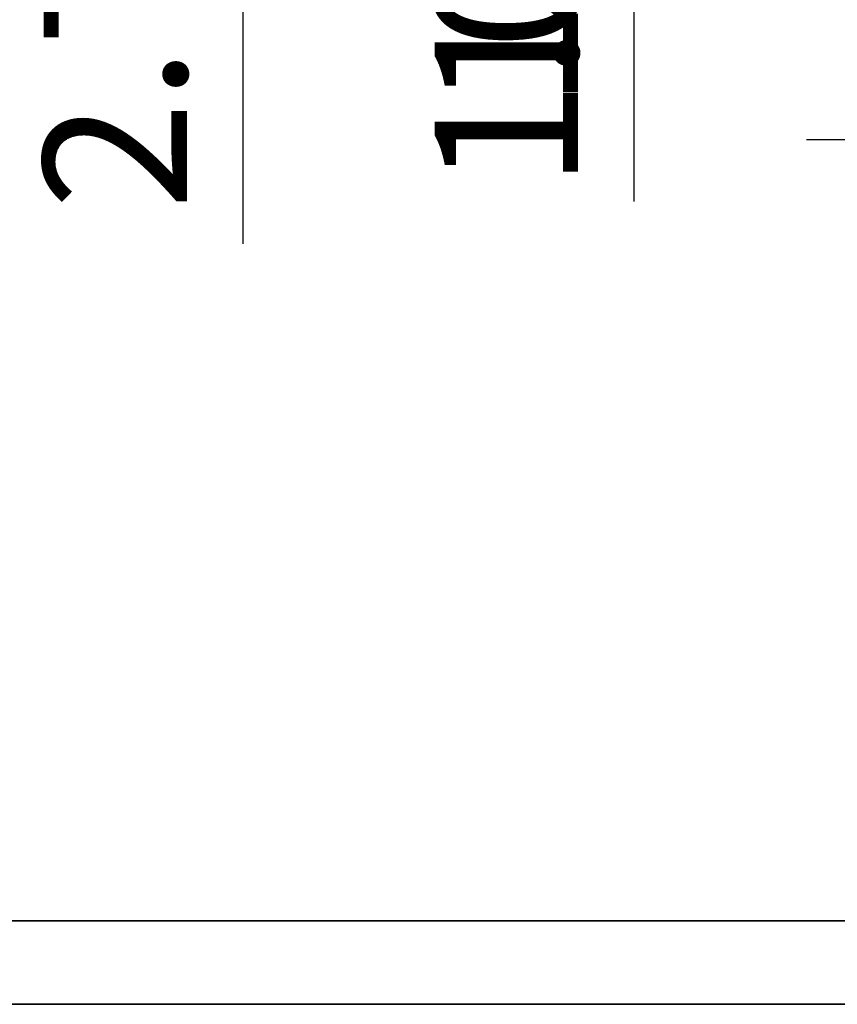
# Model space of a CAD drawing. Units: metres. Extents: x 782 to 1487, y 1262 to 7446.
# Tile 2 of 25: x 807.01 to 821.27, y 1262.35 to 1279.51. Entities that reach past the tile are written whole.
import ezdxf

# ---------------------------------------------------------------- set-up
doc = ezdxf.new("R2010")
doc.units = ezdxf.units.M
doc.layers.add('A-ANNO-DIMS', color=2, linetype='Continuous', lineweight=18)
doc.layers.add('A-ANNO-TTLB', color=7, linetype='Continuous', lineweight=35)
doc.styles.get("Standard").update_dxf_attribs({"font": 'arial.ttf'})
doc.dimstyles.new('ISO-25', dxfattribs={"dimtxt": 2.5, "dimasz": 2.5, "dimexe": 1.25, "dimexo": 0.625, "dimtad": 1, "dimtxsty": 'Standard', "dimcen": 2.5, "dimadec": 0, "dimazin": 0, "dimtfac": 1, "dimtmove": 0, "dimatfit": 3, "dimfxl": 1, "dimarcsym": 0})

# ---------------------------------------------------------------- blocks, each defined once
blk = doc.blocks.new('*D10')
at = {"layer": 'A-ANNO-DIMS', "color": 0, "lineweight": -2, "transparency": 16777216}
for p, q in [((825.73, 1277.527), (825.73, 1276.166)), ((826.753, 1277.552), (826.753, 1276.166)), ((823.23, 1277.416), (820.73, 1277.416)), ((825.73, 1277.416), (826.753, 1277.416)), ((829.253, 1277.416), (839.235, 1277.416))]:
    blk.add_line(p, q, dxfattribs=at)
at = {"layer": 'A-ANNO-DIMS', "color": 0, "transparency": 16777216}
for points in [[(823.23, 1277.833), (823.23, 1276.999), (825.73, 1277.416)], [(829.253, 1277.833), (829.253, 1276.999), (826.753, 1277.416)]]:
    blk.add_solid(points, dxfattribs=at)
at = {"layer": 'Defpoints', "color": 0, "transparency": 16777216}
for p in [(825.73, 1278.152), (826.753, 1278.177), (826.753, 1277.416)]:
    blk.add_point(p, dxfattribs=at)
at = {"layer": 'A-ANNO-DIMS', "color": 0, "transparency": 16777216, "insert": (835.494, 1279.543), "char_height": 2.5, "attachment_point": 5}
blk.add_mtext('1,02', dxfattribs=at)
blk = doc.blocks.new('*D62')
at = {"layer": 'A-ANNO-DIMS', "color": 0, "lineweight": -2, "transparency": 16777216}
for p, q in [((810.9, 1295.567), (810.9, 1298.067)), ((811.505, 1293.067), (809.65, 1293.067)), ((810.9, 1293.067), (810.9, 1290.305)), ((811.505, 1290.305), (809.65, 1290.305)), ((810.9, 1287.805), (810.9, 1275.602))]:
    blk.add_line(p, q, dxfattribs=at)
at = {"layer": 'A-ANNO-DIMS', "color": 0, "transparency": 16777216}
for points in [[(810.483, 1295.567), (811.317, 1295.567), (810.9, 1293.067)], [(810.483, 1287.805), (811.317, 1287.805), (810.9, 1290.305)]]:
    blk.add_solid(points, dxfattribs=at)
at = {"layer": 'Defpoints', "color": 0, "transparency": 16777216}
for p in [(812.13, 1293.067), (810.9, 1290.305), (812.13, 1290.305)]:
    blk.add_point(p, dxfattribs=at)
at = {"layer": 'A-ANNO-DIMS', "color": 0, "transparency": 16777216, "insert": (808.999, 1280.454), "char_height": 2.5, "attachment_point": 5, "rotation": 90}
blk.add_mtext('2.762', dxfattribs=at)
blk = doc.blocks.new('*D67')
at = {"layer": 'A-ANNO-DIMS', "color": 0, "lineweight": -2, "transparency": 16777216}
for p, q in [((817.721, 1296.199), (817.721, 1298.699)), ((817.205, 1293.699), (818.971, 1293.699)), ((817.721, 1293.699), (817.721, 1293.067)), ((817.205, 1293.067), (818.971, 1293.067)), ((817.721, 1290.567), (817.721, 1278.407))]:
    blk.add_line(p, q, dxfattribs=at)
at = {"layer": 'A-ANNO-DIMS', "color": 0, "transparency": 16777216}
for points in [[(817.304, 1296.199), (818.138, 1296.199), (817.721, 1293.699)], [(817.304, 1290.567), (818.138, 1290.567), (817.721, 1293.067)]]:
    blk.add_solid(points, dxfattribs=at)
at = {"layer": 'Defpoints', "color": 0, "transparency": 16777216}
for p in [(816.58, 1293.699), (816.58, 1293.067), (817.721, 1293.067)]:
    blk.add_point(p, dxfattribs=at)
at = {"layer": 'A-ANNO-DIMS', "color": 0, "transparency": 16777216, "insert": (815.819, 1283.237), "char_height": 2.5, "attachment_point": 5, "rotation": 90}
blk.add_mtext('0.632', dxfattribs=at)
blk = doc.blocks.new('*D68')
at = {"layer": 'A-ANNO-DIMS', "color": 0, "lineweight": -2, "transparency": 16777216}
for p, q in [((817.721, 1295.567), (817.721, 1298.067)), ((815.508, 1293.067), (818.971, 1293.067)), ((817.721, 1293.067), (817.721, 1291.686)), ((815.508, 1291.686), (818.971, 1291.686)), ((817.721, 1289.186), (817.721, 1277.718))]:
    blk.add_line(p, q, dxfattribs=at)
at = {"layer": 'A-ANNO-DIMS', "color": 0, "transparency": 16777216}
for points in [[(817.304, 1295.567), (818.138, 1295.567), (817.721, 1293.067)], [(817.304, 1289.186), (818.138, 1289.186), (817.721, 1291.686)]]:
    blk.add_solid(points, dxfattribs=at)
at = {"layer": 'Defpoints', "color": 0, "transparency": 16777216}
for p in [(814.883, 1293.067), (814.883, 1291.686), (817.721, 1291.686)]:
    blk.add_point(p, dxfattribs=at)
at = {"layer": 'A-ANNO-DIMS', "color": 0, "transparency": 16777216, "insert": (815.819, 1282.202), "char_height": 2.5, "attachment_point": 5, "rotation": 90}
blk.add_mtext('1.381', dxfattribs=at)
blk = doc.blocks.new('*D69')
at = {"layer": 'A-ANNO-DIMS', "color": 0, "lineweight": -2, "transparency": 16777216}
for p, q in [((817.721, 1294.186), (817.721, 1296.686)), ((815.508, 1291.686), (818.971, 1291.686)), ((817.721, 1291.686), (817.721, 1290.305)), ((815.508, 1290.305), (818.971, 1290.305)), ((817.721, 1287.805), (817.721, 1276.337))]:
    blk.add_line(p, q, dxfattribs=at)
at = {"layer": 'A-ANNO-DIMS', "color": 0, "transparency": 16777216}
for points in [[(817.304, 1294.186), (818.138, 1294.186), (817.721, 1291.686)], [(817.304, 1287.805), (818.138, 1287.805), (817.721, 1290.305)]]:
    blk.add_solid(points, dxfattribs=at)
at = {"layer": 'Defpoints', "color": 0, "transparency": 16777216}
for p in [(814.883, 1291.686), (814.883, 1290.305), (817.721, 1290.305)]:
    blk.add_point(p, dxfattribs=at)
at = {"layer": 'A-ANNO-DIMS', "color": 0, "transparency": 16777216, "insert": (815.819, 1280.821), "char_height": 2.5, "attachment_point": 5, "rotation": 90}
blk.add_mtext('1.381', dxfattribs=at)

msp = doc.modelspace()

# ---------------------------------------------------------------- linework, layer by layer
at = {"layer": 'A-ANNO-TTLB'}
for points in [[(787.4248, 1342.9861), (880.8003, 1342.9861), (880.8003, 1263.8004), (787.4248, 1263.8004)], [(883.6865, 1262.3458), (787.4248, 1262.3458), (787.4248, 1342.9861), (883.6865, 1342.9861)], [(788.8147, 1341.5907), (880.8003, 1341.5907), (880.8003, 1263.8004), (788.8147, 1263.8004)]]:
    msp.add_lwpolyline(points, close=True, dxfattribs=at)

# ---------------------------------------------------------------- dimensions: what is measured, and where the dimension line sits
at = {"layer": 'A-ANNO-DIMS'}
for base, p1, p2, picture, middle in [((817.7211, 1293.0674), (816.58, 1293.6994), (816.58, 1293.0674), '*D67', (815.8188, 1283.2371)), ((810.9, 1290.3053), (812.13, 1293.0674), (812.13, 1290.3053), '*D62', (808.9986, 1280.4536)), ((817.7211, 1291.6863), (814.8832, 1293.0674), (814.8832, 1291.6863), '*D68', (815.8188, 1282.2022)), ((817.7211, 1290.3053), (814.8832, 1291.6863), (814.8832, 1290.3053), '*D69', (815.8188, 1280.8211))]:
    dim = msp.add_linear_dim(base=base, p1=p1, p2=p2, angle=90, dimstyle='ISO-25', override={"dimdec": 3, "dimlfac": 1, "dimrnd": 0, "dimzin": 0, "dimdsep": 46, "dimlunit": 2}, dxfattribs=at)
    dim.commit()
    dim.dimension.update_dxf_attribs({"geometry": picture, "text_midpoint": middle})
dim = msp.add_linear_dim(base=(826.7525, 1277.4159), p1=(825.7296, 1278.1516), p2=(826.7525, 1278.177), dimstyle='ISO-25', override={"dimclrd": 0, "dimclre": 0, "dimclrt": 0}, dxfattribs=at)
dim.commit()
dim.dimension.update_dxf_attribs({"geometry": '*D10', "text_midpoint": (835.494, 1277.4159), "dimtype": 160})

doc.saveas('drawing.dxf')
